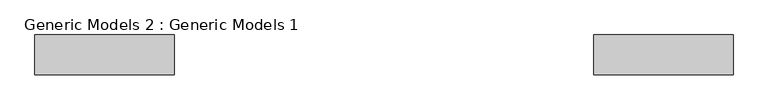
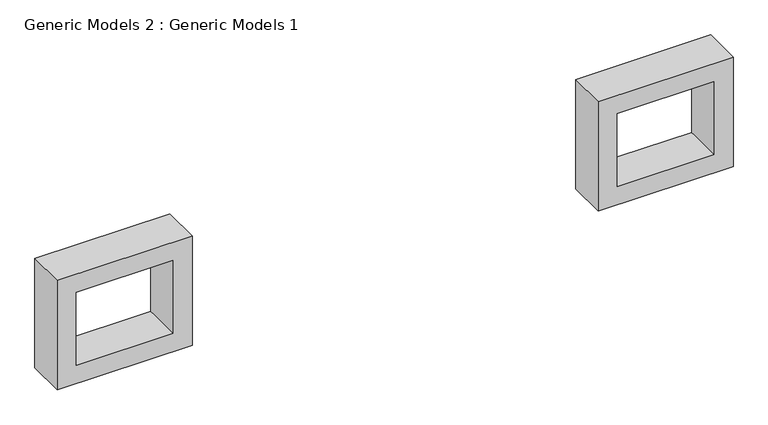
"""IFC4 building model written with IfcOpenShell, lengths in millimetres: proxy geometry, Generic Models 2 : Generic Models 1."""

from ifc_helpers import new_model, si_unit, frame, origin, place, context, project, spatial, polyline, outline, extrude, source, transform, mapped, element, save


def generic_models_2_generic_models_1_c5d0751e(model_context):
    return source(origin(), model_context, "Body", "SweptSolid", [
        extrude(outline(polyline([(8839.2, -3915.3833787), (8839.2, -6048.9833787), (7010.4, -6048.9833787), (7010.4, -3915.3833787), (8839.2, -3915.3833787)]), holes=[polyline([(8534.4, -4220.1833787), (7315.2, -4220.1833787), (7315.2, -5744.1833787), (8534.4, -5744.1833787), (8534.4, -4220.1833787)])]), frame((0.0, -10658.540066, 0.0), z_axis=(0.0, 1.0, 0.0), x_axis=(0.0, 0.0, 1.0)), (0.0, 0.0, 1.0), 609.6),
        extrude(outline(polyline([(8839.2, 4631.7166213), (8839.2, 2498.1166213), (7010.4, 2498.1166213), (7010.4, 4631.7166213), (8839.2, 4631.7166213)]), holes=[polyline([(8534.4, 4326.9166213), (7315.2, 4326.9166213), (7315.2, 2802.9166213), (8534.4, 2802.9166213), (8534.4, 4326.9166213)])]), frame((0.0, -10658.540066, 0.0), z_axis=(0.0, 1.0, 0.0), x_axis=(0.0, 0.0, 1.0)), (0.0, 0.0, 1.0), 609.6),
    ])


if __name__ == "__main__":
    model = new_model("IFC4")
    model_context = context("Model", 3, world=origin())
    ifc_project = project(units=[si_unit("LENGTHUNIT", "METRE", prefix="MILLI")], contexts=[model_context])
    site = spatial("IfcSite", under=ifc_project)
    building = spatial("IfcBuilding", under=site)
    placement = place(None, origin())
    generic_models_2_generic_models_1_shape = generic_models_2_generic_models_1_c5d0751e(model_context)
    element("IfcBuildingElementProxy", 1, Name="Generic Models 2 : Generic Models 1", ObjectType="Generic Models 2 : Generic Models 1", at=placement, inside=building, context=model_context, shape_type="MappedRepresentation", body=[
        mapped(generic_models_2_generic_models_1_shape, transform((0.0, 0.0, 0.0), x_axis=(1.0, 0.0, 0.0), y_axis=(0.0, 1.0, 0.0), z_axis=(0.0, 0.0, 1.0))),
    ])
    save(model, "model.ifc")

# Revit data of these elements
# Element 1 (IfcBuildingElementProxy, "Generic Models 2 : Generic Models 1")
#   Materials on its faces: "grey"
# Materials
#   "grey": class "Generic", colour RGB 33 34 34, transparency 0, Cost = 0
